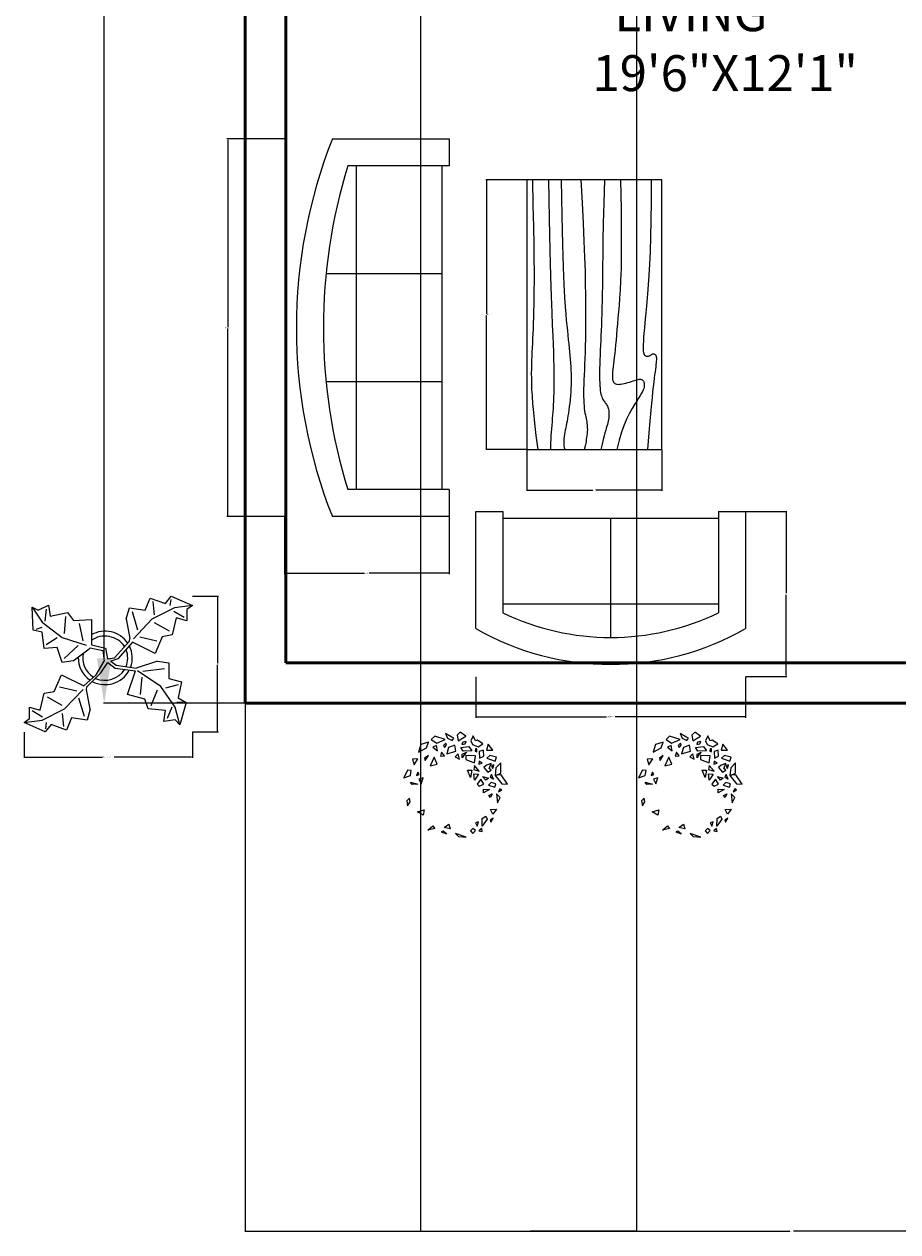
# Model space of a CAD drawing. Units: inches. Extents: x 177 to 602, y 30 to 608.
# Tile 1 of 4: x 204 to 398, y 31 to 299. Entities that reach past the tile are written whole.
import ezdxf

# ---------------------------------------------------------------- set-up
doc = ezdxf.new("R2010")
doc.units = ezdxf.units.IN
doc.header["$MEASUREMENT"] = 0
for name, color, linetype, lineweight in [('A-ANNO-DIMS', 2, 'Continuous', 18), ('A-AREA-IDEN', 7, 'Continuous', 25), ('A-FURN', 8, 'Continuous', 18), ('A-WALL', 7, 'Continuous', 50), ('L-PLNT', 94, 'Continuous', 13)]:
    doc.layers.add(name, color=color, linetype=linetype, lineweight=lineweight)
doc.styles.get("Standard").update_dxf_attribs({"font": 'arial.ttf'})
doc.dimstyles.get("Standard").update_dxf_attribs({"dimtxt": 0.18, "dimasz": 0.18, "dimexe": 0.18, "dimexo": 0.0625, "dimgap": 0.09, "dimtad": 0, "dimtih": 1, "dimtoh": 1, "dimdec": 1, "dimzin": 0, "dimdsep": 46, "dimlunit": 4, "dimtxsty": 'Standard', "dimcen": 0.09, "dimadec": 0, "dimazin": 0, "dimtfac": 1, "dimtdec": 1, "dimtofl": 0, "dimtmove": 0, "dimatfit": 3, "dimfxl": 1, "dimtolj": 1, "dimtzin": 0, "dimarcsym": 0})

# ---------------------------------------------------------------- blocks, each defined once
blk = doc.blocks.new('*U9')
for points in [[(-4.43, 11.05), (-5.18, 10.36), (-3.96, 9.49), (-2.07, 10.36)], [(-2, 11.66), (-1.6, 10.62), (-0.52, 10.1), (-0.18, 10.62), (-0.79, 10.96)], [(1.24, 12), (0.56, 11.31), (0.76, 10.01), (2.52, 11.05)], [(4.14, 11.14), (3.6, 10.01), (4, 9.23), (5.22, 8.71), (6.3, 9.41), (5.08, 10.19), (4.61, 10.01)], [(-5.78, 9.75), (-7.54, 9.23), (-8.01, 7.5), (-6.26, 8.45)], [(-4.84, 8.63), (-3.83, 7.85), (-4.03, 8.97)], [(-1.94, 9.49), (-2.48, 8.97), (-2.27, 8.54), (-1.8, 9.06)], [(0.02, 9.06), (-1.33, 8.54), (-1.73, 7.16), (0.29, 7.76)], [(1.37, 8.54), (3.13, 8.8), (3.8, 7.85), (1.91, 7.76)], [(2.59, 9.93), (1.84, 9.75), (1.64, 9.23), (2.32, 9.41)], [(4.61, 8.28), (4.54, 7.76), (4.95, 7.59), (4.95, 8.28)], [(7.45, 9.32), (7.11, 7.94), (8.52, 7.94)], [(-8.14, 6.03), (-9.36, 5.95), (-9.02, 4.73)], [(-5.78, 6.81), (-6.66, 6.21), (-6.52, 5.69)], [(-4.57, 6.38), (-5.45, 4.47), (-3.89, 4.82)], [(-2.88, 7.5), (-3.15, 6.64), (-2.27, 6.72)], [(0.76, 7.16), (0.09, 6.46), (1.1, 5.95)], [(1.71, 6.29), (1.71, 7.07), (2.65, 7.5), (2.11, 6.9)], [(2.52, 6.81), (2.52, 5.86), (4.41, 5.17), (4.61, 6.72)], [(5.49, 5.51), (5.42, 4.82), (6.16, 5.08)], [(6.43, 7.94), (5.49, 7.68), (5.56, 6.21), (6.5, 6.64)], [(7.85, 6.81), (7.18, 6.21), (9, 5.51), (9.33, 6.38)], [(-11.32, 1.79), (-9.83, 2.31), (-9.63, 3.44), (-10.44, 3.52)], [(-8.21, 3.09), (-8.48, 2.31), (-7.87, 2.57)], [(3.53, 1.88), (2.86, 3.52), (3.8, 3.52)], [(4.41, 4.56), (4.27, 3.7), (5.49, 3.26)], [(4.27, 2.74), (5.29, 2.66), (4.41, 1.27)], [(8.12, 4.99), (7.11, 4.65), (6.5, 4.13), (7.38, 3.09), (8.12, 3.52), (7.65, 3.87)], [(8.73, 4.73), (8.19, 4.56), (8.39, 3.87), (8.59, 4.04)], [(10.28, 5.17), (9.2, 4.04), (9, 2.31), (10.48, 0.49), (11.76, 0.41), (10.35, 2.48), (9.33, 2.4), (10.28, 2.83)], [(-8.21, 0.41), (-9.43, 0.32), (-9.83, 0.84)], [(-7, 1.79), (-7.94, 1.53), (-7.47, 0.49)], [(5.83, 1.53), (5.02, 0.41), (5.49, -0.02), (6.5, 0.41)], [(7.51, 1.71), (6.91, 1.27), (6.23, 2.14)], [(8.12, 0.75), (7.51, 0.15), (8.93, -0.28), (9.13, 0.49)], [(8.19, 2.57), (7.92, 2.05), (8.66, 1.53)], [(7.78, -0.8), (6.43, -1.5), (6.43, -0.72)], [(8.32, -1.75), (7.98, -2.53), (7.58, -2.1)], [(9.33, -1.75), (9.54, -3.74), (10.14, -2.53)], [(10.08, -0.63), (9.74, -1.32), (10.48, -0.89)], [(-10.03, -2.71), (-10.64, -3.31), (-10.44, -4.44), (-9.9, -3.49)], [(-8.28, -5.73), (-6.79, -5.3), (-7, -6.51)], [(9.33, -5.13), (8.46, -6.25), (7.98, -5.22)], [(5.29, -7.98), (4.61, -8.16), (5.02, -8.94)], [(6.1, -8.94), (6.16, -7.21), (6.91, -6.69), (7.24, -7.38)], [(8.05, -8.07), (8.59, -7.12), (7.92, -7.55)], [(-4.84, -8.85), (-4.43, -9.45), (-5.99, -9.8)], [(-2.54, -10.06), (-3.02, -10.23), (-1.8, -10.67)], [(-2.34, -9.2), (-1.26, -8.5), (-0.99, -9.54)], [(0.22, -10.58), (0.83, -11.27), (2.59, -11.36)], [(4.07, -9.45), (3.53, -9.97), (4.07, -10.58), (4.61, -9.89)], [(6.03, -9.45), (5.42, -9.97), (6.16, -10.15)]]:
    blk.add_lwpolyline(points, close=True)
blk = doc.blocks.new('Sofa - Roundback 7 ft.')
for p, q in [((-12.00002, -32.4421), (-12.00003, -6.5971)), ((11.99997, -32.4421), (11.99998, -6.5971)), ((-36.000027, -34), (-36.000027, -11.4696)), ((-35.999844, -13.3819), (35.9998, -13.3819)), ((35.99998, -34), (35.99998, -11.4696)), ((-36.000027, -32.4421), (35.99998, -32.4421))]:
    blk.add_line(p, q)
for points in [[(-36.000027, -34), (-42.000027, -34), (-42.000027, -8)], [(41.99998, -8), (41.99998, -34), (35.99998, -34)]]:
    blk.add_lwpolyline(points)
for centre, radius, start, end in [((0, -114.25), 114.25, 68.43141, 111.5686), ((-0.00001, -127.1968), 121.1968, 72.72033, 107.2797)]:
    blk.add_arc(centre, radius, start, end)
blk = doc.blocks.new('Sofa - Roundback Loveseat 5 ft.')
for p, q in [((0, -32.44198), (0, -5.99998)), ((-24, -33.99998), (-24, -11.46958)), ((-23.9998, -13.38178), (23.99986, -13.38178)), ((24.00004, -33.99998), (24.00004, -11.46958)), ((-24, -32.44198), (24.00004, -32.44198))]:
    blk.add_line(p, q)
for points in [[(-24, -33.99998), (-30, -33.99998), (-30, -7.99998)], [(30.00004, -7.99998), (30.00004, -33.99998), (24.00004, -33.99998)]]:
    blk.add_lwpolyline(points)
for centre, radius, start, end in [((0, -60.24998), 60.24998, 60.13715, 119.8628), ((0, -61.38438), 55.38444, 64.32083, 115.6792)]:
    blk.add_arc(centre, radius, start, end)
blk = doc.blocks.new('Plant - Rubber or Philodendron')
for p, q in [((8.8871, 10.7908), (9.9809, 13.4933)), ((9.9809, 13.4933), (13.3837, 12.301)), ((13.3837, 12.301), (14.68, 13.9039)), ((14.68, 13.9039), (19.3848, 11.8146)), ((-16.2005, 11.4774), (-13.9899, 8.1064)), ((-16.2005, 11.4774), (-14.8639, 10.7964)), ((-16.0159, 6.3329), (-16.2005, 11.4774)), ((-14.8639, 10.7964), (-12.6195, 11.8975)), ((-13.3174, 8.325), (-13.0735, 11.0065)), ((-12.6195, 11.8975), (-12.1909, 9.4345)), ((4.6914, 8.8812), (5.3859, 11.2828)), ((5.3859, 11.2828), (8.8871, 10.7908)), ((15.3859, 11.3055), (10.3916, 8.7942)), ((10.5828, 12.6946), (10.8893, 9.7953)), ((14.5816, 13.2037), (14.3848, 11.8033)), ((19.3848, 11.8146), (15.3859, 11.3055)), ((19.3848, 11.8146), (18.1868, 10.9119)), ((18.1868, 10.9119), (18.1925, 8.4119)), ((-13.9899, 8.1064), (-9.5434, 4.7185)), ((-12.1909, 9.4345), (-8.3829, 10.3)), ((-8.8369, 9.409), (-9.0894, 5.6095)), ((-8.3829, 10.3), (-7.0549, 8.501)), ((-7.0549, 8.501), (-3.0284, 8.6941)), ((-3.0284, 8.6941), (-3.0709, 3.1041)), ((4.6914, 8.8812), (5.5014, 4.4831)), ((5.9878, 10.4842), (7.1971, 6.3869)), ((10.3916, 8.7942), (6.2847, 4.4028)), ((15.7909, 9.1065), (14.8995, 5.3044)), ((15.2875, 10.6053), (17.5907, 9.2105)), ((18.1925, 8.4119), (15.7909, 9.1065)), ((-14.0069, 5.8704), (-16.0159, 6.3329)), ((-15.3434, 6.5514), (-13.9984, 6.9884)), ((-13.5868, 2.2894), (-14.0069, 5.8704)), ((-4.8529, 4.012), (-5.7184, 7.82)), ((14.2977, 6.1031), (10.9934, 7.9956)), ((-13.1329, 3.1804), (-10.6614, 4.727)), ((-9.5434, 4.7185), (-4.1917, 2.9888)), ((-9.1318, 0.0195), (-5.9793, 2.9025)), ((-3.0709, 3.1041), (0.0797, 2.3163)), ((2.1141, 0.2298), (5.4346, 3.9146)), ((6.1032, 3.6844), (2.8262, -0.031)), ((5.4346, 3.9146), (5.5014, 4.4831)), ((11.1089, 1.1958), (6.1032, 3.6844)), ((7.7005, 4.8881), (11.5025, 3.9967)), ((12.7005, 4.8994), (11.1089, 1.1958)), ((14.8995, 5.3044), (12.7005, 4.8994)), ((-10.6784, 2.491), (-13.5868, 2.2894)), ((-9.5858, -0.8715), (-10.6784, 2.491)), ((-7.1228, -0.443), (-3.5248, 2.2131)), ((-3.5248, 2.2131), (-3.3011, 2.4355)), ((-3.3011, 2.4355), (-0.5306, 1.7947)), ((-0.5306, 1.7947), (-0.2255, -0.5527)), ((-0.5306, 1.7947), (-0.5306, 1.7947)), ((0.0797, 2.3163), (0.4866, -0.031)), ((0.4866, -0.031), (2.1141, 0.2298)), ((-7.1228, -0.443), (-9.5858, -0.8715)), ((-2.019, -3.6148), (-0.2255, -0.5527)), ((-0.9375, -3.1608), (0.5883, -0.8135)), ((0.5883, -0.8135), (2.2447, -2.0916)), ((2.8262, -0.031), (1.3003, -0.5527)), ((1.3003, -0.5527), (2.4193, -1.4655)), ((2.2447, -2.0916), (6.7108, -2.6626)), ((2.4193, -1.4655), (6.895, -2.1175)), ((4.943, -7.9659), (6.7108, -2.6626)), ((11.6605, -0.5413), (6.895, -2.1175)), ((12.3677, -6.1981), (7.219, -2.6772)), ((8.3544, -2.7453), (13.1973, -2.1704)), ((11.6605, -0.5413), (14.1354, -0.8948)), ((14.1354, -0.8948), (14.1354, -4.4304)), ((-11.3237, -7.2629), (-9.7321, -3.5593)), ((-9.7321, -3.5593), (-4.7264, -6.0479)), ((-2.019, -3.6148), (-4.7264, -6.0479)), ((-4.0579, -6.2781), (-0.9375, -3.1608)), ((8.125, -4.0768), (7.7715, -7.9659)), ((14.1354, -4.4304), (16.9638, -5.1375)), ((16.9638, -5.1375), (16.2567, -8.673)), ((-14.4141, -11.4699), (-13.5228, -7.6679)), ((-13.5228, -7.6679), (-11.3237, -7.2629)), ((-6.3237, -7.2516), (-10.1257, -6.3602)), ((-9.0148, -11.1577), (-4.9047, -6.8122)), ((-4.1246, -6.8466), (-4.0579, -6.2781)), ((-3.3146, -11.2447), (-4.1246, -6.8466)), ((8.8321, -9.0266), (4.943, -7.9659)), ((10.2463, -10.4408), (11.6605, -6.9053)), ((15.5496, -10.7943), (12.3677, -6.1981)), ((16.2567, -5.8446), (13.4283, -6.5517)), ((-12.921, -8.4665), (-9.6166, -10.359)), ((-4.611, -12.8477), (-5.8203, -8.7504)), ((9.5392, -11.1479), (8.8321, -9.0266)), ((17.3174, -9.7337), (15.9032, -9.7337)), ((16.2567, -8.673), (18.0245, -9.7337)), ((18.0245, -9.7337), (16.6103, -14.6834)), ((-18.008, -14.1781), (-16.8101, -13.2754)), ((-16.8157, -10.7754), (-14.4141, -11.4699)), ((-16.8101, -13.2754), (-16.8157, -10.7754)), ((-13.9107, -12.9688), (-16.2139, -11.574)), ((-14.0091, -13.669), (-9.0148, -11.1577)), ((-9.206, -15.0581), (-9.5126, -12.1588)), ((-7.5103, -13.1543), (-8.6042, -15.8568)), ((-4.0092, -13.6463), (-7.5103, -13.1543)), ((-3.3146, -11.2447), (-4.0092, -13.6463)), ((13.4283, -11.5015), (9.5392, -11.1479)), ((13.0748, -13.9763), (13.4283, -11.5015)), ((14.8425, -10.7943), (13.7819, -13.2692)), ((16.6103, -14.6834), (15.5496, -10.7943)), ((-18.008, -14.1781), (-14.0091, -13.669)), ((-13.3032, -16.2674), (-18.008, -14.1781)), ((-12.0069, -14.6645), (-13.3032, -16.2674)), ((-13.2048, -15.5672), (-13.008, -14.1668)), ((-8.6042, -15.8568), (-12.0069, -14.6645)), ((15.5496, -13.6228), (13.0748, -13.9763)), ((16.6103, -14.6834), (15.5496, -13.6228))]:
    blk.add_line(p, q)
for centre, radius, start, end in [((0, 0), 6.1275, 34.37569, 120.1028), ((-0.0601, -0.2075), 5.2461, 33.82192, 124.9414), ((-0.098, 0.1364), 6.1288, 341.2017, 26.09184), ((0.0308, 0.1664), 6, 178.6147, 235.1169), ((0.0308, 0.1664), 5, 168.1647, 238.6725), ((-0.2664, 0.1682), 5.2775, 338.4094, 20.03007), ((-0.0234, 0.3825), 6.1492, 242.5812, 331.2714), ((-0.1102, 0.4886), 5.2883, 247.3711, 327.472)]:
    blk.add_arc(centre, radius, start, end)
blk = doc.blocks.new('Table - Rectangular Woodgrain 60 x 30 in.')
for p, q in [((0, 0), (0, -30)), ((60, 0), (0, 0)), ((60, -30), (60, 0)), ((0, -30), (60, -30))]:
    blk.add_line(p, q)
for points in [[(0, -2.4), (4.8155, -2.418), (9.0302, -2.4688), (12.709, -2.5477), (15.9167, -2.65), (18.7181, -2.7711), (21.1781, -2.9063), (23.3616, -3.0508), (25.3333, -3.2), (27.1477, -3.3495), (28.8172, -3.4958), (30.3437, -3.636), (31.7291, -3.7667), (32.9756, -3.8849), (34.0849, -3.9875), (35.059, -4.0714), (35.9, -4.1334), (36.6114, -4.1711), (37.2041, -4.1854), (37.6906, -4.1779), (38.0833, -4.15), (38.3948, -4.1034), (38.6375, -4.0396), (38.8239, -3.9602), (38.9666, -3.8667), (39.0764, -3.7608), (39.1573, -3.6448), (39.2116, -3.521), (39.2416, -3.3917), (39.2498, -3.2593), (39.2385, -3.1261), (39.21, -2.9944), (39.1666, -2.8667), (39.111, -2.7447), (39.0468, -2.6281), (38.978, -2.5163), (38.9083, -2.4083), (38.8418, -2.3035), (38.7823, -2.201), (38.7337, -2.1001), (38.7, -2), (38.6844, -1.9003), (38.6875, -1.8021), (38.7094, -1.707), (38.75, -1.6167), (38.8094, -1.5326), (38.8875, -1.4563), (38.9844, -1.3893), (39.1, -1.3333), (39.2351, -1.2896), (39.3937, -1.2583), (39.5804, -1.2396), (39.8, -1.2333), (40.057, -1.2396), (40.3562, -1.2583), (40.7023, -1.2896), (41.1, -1.3333), (41.5547, -1.3895), (42.0755, -1.4573), (42.6721, -1.5361), (43.3542, -1.625), (44.1316, -1.7233), (45.014, -1.8302), (46.0114, -1.9449), (47.1333, -2.0667), (48.3862, -2.1947), (49.7625, -2.3281), (51.2513, -2.4663), (52.8416, -2.6083), (54.5226, -2.7535), (56.2833, -2.9011), (58.1127, -3.0501), (60, -3.2)], [(0, -9.2), (6.5759, -9.0858), (11.9385, -9.0365), (16.2527, -9.0418), (19.6833, -9.0917), (22.3952, -9.1759), (24.5531, -9.2844), (26.322, -9.4069), (27.8666, -9.5333), (29.3241, -9.6553), (30.7203, -9.7719), (32.0532, -9.8837), (33.3208, -9.9917), (34.5213, -10.0965), (35.6526, -10.199), (36.7128, -10.2999), (37.7, -10.4), (38.6129, -10.4996), (39.4531, -10.5969), (40.223, -10.6895), (40.925, -10.775), (41.5613, -10.8512), (42.1344, -10.9156), (42.6465, -10.966), (43.1, -11), (43.4976, -11.0158), (43.8437, -11.0136), (44.143, -10.9942), (44.4, -10.9583), (44.6195, -10.9069), (44.8062, -10.8406), (44.9648, -10.7603), (45.1, -10.6667), (45.2155, -10.5598), (45.3114, -10.4365), (45.3871, -10.2929), (45.4416, -10.125), (45.4743, -9.929), (45.4844, -9.7011), (45.4709, -9.4371), (45.4333, -9.1333), (45.3716, -8.7883), (45.2896, -8.4104), (45.1919, -8.0107), (45.0833, -7.6), (44.9685, -7.1893), (44.8521, -6.7896), (44.7388, -6.4117), (44.6333, -6.0667), (44.54, -5.7628), (44.4614, -5.4979), (44.4001, -5.2675), (44.3583, -5.0667), (44.3384, -4.8909), (44.3427, -4.7354), (44.3736, -4.5956), (44.4333, -4.4667), (44.5236, -4.3453), (44.6427, -4.2333), (44.7884, -4.1339), (44.9583, -4.05), (45.1501, -3.9849), (45.3614, -3.9417), (45.59, -3.9234), (45.8333, -3.9333), (46.0915, -3.9749), (46.3734, -4.0531), (46.6906, -4.1736), (47.0542, -4.3417), (47.4756, -4.5629), (47.9661, -4.8427), (48.5372, -5.1866), (49.2, -5.6), (49.9676, -6.0844), (50.8594, -6.625), (51.8965, -7.2031), (53.1, -7.8), (54.491, -8.3969), (56.0906, -8.975), (57.9199, -9.5156), (60, -10)], [(0, -12.8), (5.1847, -12.9322), (9.6213, -13.0323), (13.3963, -13.1059), (16.5958, -13.1583), (19.3063, -13.1952), (21.614, -13.2219), (23.6054, -13.2439), (25.3666, -13.2667), (26.9728, -13.2947), (28.4531, -13.3281), (29.8256, -13.3663), (31.1083, -13.4083), (32.3191, -13.4535), (33.476, -13.501), (34.597, -13.5501), (35.7, -13.6), (36.7984, -13.6497), (37.8875, -13.6979), (38.9578, -13.743), (40, -13.7833), (41.0047, -13.8174), (41.9625, -13.8438), (42.864, -13.8607), (43.7, -13.8667), (44.4631, -13.8604), (45.1552, -13.8417), (45.7801, -13.8104), (46.3416, -13.7667), (46.8439, -13.7104), (47.2906, -13.6417), (47.6858, -13.5604), (48.0333, -13.4667), (48.3375, -13.3608), (48.6042, -13.2448), (48.8396, -13.121), (49.05, -12.9917), (49.2417, -12.8593), (49.4208, -12.7261), (49.5937, -12.5944), (49.7667, -12.4667), (49.9452, -12.3451), (50.1323, -12.2313), (50.3303, -12.1268), (50.5416, -12.0333), (50.7686, -11.9524), (51.0135, -11.8854), (51.2788, -11.8341), (51.5666, -11.8), (51.8785, -11.7843), (52.2116, -11.7865), (52.562, -11.8059), (52.926, -11.8417), (53.2998, -11.8931), (53.6795, -11.9594), (54.0614, -12.0397), (54.4416, -12.1333), (54.8223, -12.2401), (55.2293, -12.3625), (55.6942, -12.5037), (56.2489, -12.6667), (56.9251, -12.8547), (57.7545, -13.0708), (58.7689, -13.3182), (60, -13.6)], [(0, -18), (5.124, -17.7273), (9.6609, -17.5057), (13.6705, -17.3303), (17.2125, -17.1958), (20.3467, -17.0973), (23.1328, -17.0297), (25.6307, -16.9878), (27.9, -16.9667), (29.9928, -16.9617), (31.9302, -16.9703), (33.7254, -16.9907), (35.3917, -17.0208), (36.9423, -17.0588), (38.3906, -17.1026), (39.7499, -17.1503), (41.0333, -17.2), (42.2519, -17.2496), (43.4073, -17.2969), (44.4986, -17.3395), (45.525, -17.375), (46.4858, -17.4012), (47.3802, -17.4156), (48.2074, -17.416), (48.9667, -17.4), (49.6583, -17.3662), (50.2872, -17.3167), (50.8595, -17.2547), (51.3812, -17.1833), (51.8584, -17.1057), (52.2971, -17.025), (52.7034, -16.9443), (53.0833, -16.8667), (53.443, -16.7951), (53.789, -16.7313), (54.128, -16.6768), (54.4666, -16.6334), (54.8115, -16.6024), (55.1693, -16.5854), (55.5465, -16.5841), (55.95, -16.6), (56.3828, -16.6337), (56.8346, -16.6823), (57.2915, -16.7418), (57.7396, -16.8084), (58.165, -16.878), (58.5539, -16.9469), (58.8924, -17.0111), (59.1666, -17.0667), (59.3679, -17.1107), (59.5078, -17.1438), (59.6032, -17.1675), (59.6708, -17.1833), (59.7275, -17.193), (59.7901, -17.1979), (59.8753, -17.1998), (60, -17.2)], [(0, -22.4), (8.0098, -22.2501), (14.4094, -22.1011), (19.4168, -21.9535), (23.25, -21.8083), (26.1269, -21.6663), (28.2656, -21.5281), (29.884, -21.3947), (31.2, -21.2667), (32.3967, -21.1448), (33.5172, -21.0292), (34.5697, -20.9198), (35.5625, -20.8167), (36.5037, -20.7198), (37.4015, -20.6292), (38.2642, -20.5448), (39.1, -20.4667), (39.9164, -20.3951), (40.7187, -20.3313), (41.5117, -20.2768), (42.3, -20.2333), (43.0883, -20.2024), (43.8812, -20.1854), (44.6836, -20.1841), (45.5, -20.2), (46.3328, -20.234), (47.1747, -20.2844), (48.0163, -20.3488), (48.8479, -20.425), (49.66, -20.5106), (50.4429, -20.6031), (51.1872, -20.7004), (51.8833, -20.8), (52.5246, -20.8999), (53.1166, -20.9995), (53.6681, -21.0983), (54.1875, -21.1958), (54.6834, -21.2919), (55.1646, -21.3859), (55.6394, -21.4777), (56.1167, -21.5667), (56.6028, -21.6515), (57.0961, -21.7266), (57.5929, -21.7852), (58.0896, -21.8208), (58.5823, -21.8268), (59.0674, -21.7964), (59.5412, -21.723), (60, -21.6)], [(0, -25.2), (8.6355, -25.0504), (15.7026, -24.9031), (21.4049, -24.7606), (25.9458, -24.625), (29.529, -24.4988), (32.3578, -24.3844), (34.6359, -24.284), (36.5667, -24.2), (38.3213, -24.1341), (39.9417, -24.0854), (41.437, -24.0523), (42.8167, -24.0333), (44.0901, -24.0268), (45.2667, -24.0313), (46.3557, -24.0451), (47.3667, -24.0667), (48.309, -24.0947), (49.1928, -24.1287), (50.0284, -24.168), (50.826, -24.2125), (51.5959, -24.2617), (52.3483, -24.3151), (53.0935, -24.3725), (53.8417, -24.4334), (54.6009, -24.497), (55.3699, -24.561), (56.1454, -24.6226), (56.9239, -24.6792), (57.7021, -24.7279), (58.4764, -24.7662), (59.2435, -24.7911), (60, -24.8)], [(0, -28.8), (5.6867, -28.6681), (10.45, -28.5698), (14.407, -28.5012), (17.675, -28.4584), (20.3711, -28.4374), (22.6125, -28.4344), (24.5164, -28.4455), (26.2, -28.4667), (27.762, -28.4947), (29.2276, -28.5281), (30.6033, -28.5663), (31.8958, -28.6084), (33.1118, -28.6535), (34.2578, -28.7011), (35.3405, -28.7501), (36.3666, -28.8), (37.3443, -28.8497), (38.288, -28.8974), (39.2137, -28.9412), (40.1375, -28.9792), (41.0753, -29.0093), (42.0432, -29.0297), (43.0572, -29.0384), (44.1333, -29.0333), (45.2936, -29.0114), (46.5843, -28.9641), (48.0579, -28.8816), (49.7666, -28.7542), (51.7629, -28.5721), (54.0989, -28.3255), (56.8272, -28.0048), (60, -27.6)]]:
    blk.add_lwpolyline(points)
blk = doc.blocks.new('*D33')
at = {"layer": 'A-ANNO-DIMS', "color": 0, "lineweight": -2, "transparency": 16777216}
for p, q in [((253.28, 556.14), (221.81, 556.14)), ((221.99, 546.14), (221.99, 358.36)), ((221.99, 158.14), (221.99, 345.92)), ((253.28, 148.14), (221.81, 148.14))]:
    blk.add_line(p, q, dxfattribs=at)
at = {"layer": 'A-ANNO-DIMS', "color": 0, "transparency": 16777216}
for points in [[(220.33, 546.14), (223.66, 546.14), (221.99, 556.14)], [(220.33, 158.14), (223.66, 158.14), (221.99, 148.14)]]:
    blk.add_solid(points, dxfattribs=at)
at = {"layer": 'Defpoints', "color": 0, "transparency": 16777216}
for p in [(221.99, 556.14), (253.34, 556.14), (253.34, 148.14)]:
    blk.add_point(p, dxfattribs=at)
at = {"layer": 'A-ANNO-DIMS', "color": 0, "transparency": 16777216, "insert": (221.99, 352.14), "char_height": 12, "attachment_point": 5}
blk.add_mtext("\\A1;34'", dxfattribs=at)
blk = doc.blocks.new('*D41')
at = {"layer": 'A-ANNO-DIMS', "color": 0, "lineweight": -2, "transparency": 16777216}
for p, q in [((204.2, 141.69), (204.2, 135.96)), ((241.59, 141.69), (241.59, 135.96)), ((204.38, 136.14), (221.61, 136.14)), ((241.41, 136.14), (224.18, 136.14))]:
    blk.add_line(p, q, dxfattribs=at)
at = {"layer": 'A-ANNO-DIMS', "color": 0, "transparency": 16777216}
for points in [[(204.38, 136.17), (204.38, 136.11), (204.2, 136.14)], [(241.41, 136.17), (241.41, 136.11), (241.59, 136.14)]]:
    blk.add_solid(points, dxfattribs=at)
at = {"layer": 'Defpoints', "color": 0, "transparency": 16777216}
for p in [(204.2, 141.75), (241.59, 141.75), (241.59, 136.14)]:
    blk.add_point(p, dxfattribs=at)
at = {"layer": 'A-ANNO-DIMS', "color": 0, "transparency": 16777216, "insert": (222.89, 136.14), "char_height": 0.18, "attachment_point": 5}
blk.add_mtext('\\A1;PLANT 3\'-1 1/2" TYP.', dxfattribs=at)
blk = doc.blocks.new('*D42')
at = {"layer": 'A-ANNO-DIMS', "color": 0, "lineweight": -2, "transparency": 16777216}
for p, q in [((241.65, 171.92), (247.38, 171.92)), ((247.2, 171.74), (247.2, 157.02)), ((247.2, 141.93), (247.2, 156.65)), ((241.65, 141.75), (247.38, 141.75))]:
    blk.add_line(p, q, dxfattribs=at)
at = {"layer": 'A-ANNO-DIMS', "color": 0, "transparency": 16777216}
for points in [[(247.17, 171.74), (247.23, 171.74), (247.2, 171.92)], [(247.17, 141.93), (247.23, 141.93), (247.2, 141.75)]]:
    blk.add_solid(points, dxfattribs=at)
at = {"layer": 'Defpoints', "color": 0, "transparency": 16777216}
for p in [(241.59, 171.92), (247.2, 171.92), (241.59, 141.75)]:
    blk.add_point(p, dxfattribs=at)
at = {"layer": 'A-ANNO-DIMS', "color": 0, "transparency": 16777216, "insert": (247.2, 156.84), "char_height": 0.18, "attachment_point": 5}
blk.add_mtext('\\A1;2\'-6" TYP.', dxfattribs=at)
blk = doc.blocks.new('*D57')
at = {"layer": 'A-ANNO-DIMS', "color": 0, "lineweight": -2, "transparency": 16777216}
for p, q in [((261.98, 273.62), (249.26, 273.62)), ((249.44, 273.44), (249.44, 231.8)), ((249.44, 189.8), (249.44, 231.43)), ((261.98, 189.62), (249.26, 189.62))]:
    blk.add_line(p, q, dxfattribs=at)
at = {"layer": 'A-ANNO-DIMS', "color": 0, "transparency": 16777216}
for points in [[(249.41, 273.44), (249.47, 273.44), (249.44, 273.62)], [(249.41, 189.8), (249.47, 189.8), (249.44, 189.62)]]:
    blk.add_solid(points, dxfattribs=at)
at = {"layer": 'Defpoints', "color": 0, "transparency": 16777216}
for p in [(249.44, 273.62), (262.04, 273.62), (262.04, 189.62)]:
    blk.add_point(p, dxfattribs=at)
at = {"layer": 'A-ANNO-DIMS', "color": 0, "transparency": 16777216, "insert": (249.44, 231.62), "char_height": 0.18, "attachment_point": 5}
blk.add_mtext('\\A1;SOFA 7\'-0"', dxfattribs=at)
blk = doc.blocks.new('*D58')
at = {"layer": 'A-ANNO-DIMS', "color": 0, "lineweight": -2, "transparency": 16777216}
for p, q in [((262.04, 189.55), (262.04, 176.84)), ((298.71, 189.55), (298.71, 176.84)), ((262.22, 177.02), (279.84, 177.02)), ((298.53, 177.02), (280.92, 177.02))]:
    blk.add_line(p, q, dxfattribs=at)
at = {"layer": 'A-ANNO-DIMS', "color": 0, "transparency": 16777216}
for points in [[(262.22, 177.05), (262.22, 176.99), (262.04, 177.02)], [(298.53, 177.05), (298.53, 176.99), (298.71, 177.02)]]:
    blk.add_solid(points, dxfattribs=at)
at = {"layer": 'Defpoints', "color": 0, "transparency": 16777216}
for p in [(262.04, 189.62), (298.71, 189.62), (262.04, 177.02)]:
    blk.add_point(p, dxfattribs=at)
at = {"layer": 'A-ANNO-DIMS', "color": 0, "transparency": 16777216, "insert": (280.38, 177.02), "char_height": 0.18, "attachment_point": 5}
blk.add_mtext('\\A1;3\'-0 1/2"', dxfattribs=at)
blk = doc.blocks.new('*D59')
at = {"layer": 'A-ANNO-DIMS', "color": 0, "lineweight": -2, "transparency": 16777216}
for p, q in [((304.58, 154.02), (304.58, 144.9)), ((364.58, 154.02), (364.58, 144.9)), ((304.76, 145.08), (333.56, 145.08)), ((364.4, 145.08), (335.61, 145.08))]:
    blk.add_line(p, q, dxfattribs=at)
at = {"layer": 'A-ANNO-DIMS', "color": 0, "transparency": 16777216}
for points in [[(304.76, 145.11), (304.76, 145.05), (304.58, 145.08)], [(364.4, 145.11), (364.4, 145.05), (364.58, 145.08)]]:
    blk.add_solid(points, dxfattribs=at)
at = {"layer": 'Defpoints', "color": 0, "transparency": 16777216}
for p in [(304.58, 154.08), (364.58, 154.08), (304.58, 145.08)]:
    blk.add_point(p, dxfattribs=at)
at = {"layer": 'A-ANNO-DIMS', "color": 0, "transparency": 16777216, "insert": (334.58, 145.08), "char_height": 0.18, "attachment_point": 5}
blk.add_mtext('\\A1;LOVESEAT 5\'-0"', dxfattribs=at)
blk = doc.blocks.new('*D60')
at = {"layer": 'A-ANNO-DIMS', "color": 0, "lineweight": -2, "transparency": 16777216}
for p, q in [((364.65, 190.75), (373.76, 190.75)), ((373.58, 190.57), (373.58, 172.6)), ((373.58, 154.26), (373.58, 172.23)), ((364.65, 154.08), (373.76, 154.08))]:
    blk.add_line(p, q, dxfattribs=at)
at = {"layer": 'A-ANNO-DIMS', "color": 0, "transparency": 16777216}
for points in [[(373.55, 190.57), (373.61, 190.57), (373.58, 190.75)], [(373.55, 154.26), (373.61, 154.26), (373.58, 154.08)]]:
    blk.add_solid(points, dxfattribs=at)
at = {"layer": 'Defpoints', "color": 0, "transparency": 16777216}
for p in [(364.58, 190.75), (364.58, 154.08), (373.58, 154.08)]:
    blk.add_point(p, dxfattribs=at)
at = {"layer": 'A-ANNO-DIMS', "color": 0, "transparency": 16777216, "insert": (373.58, 172.41), "char_height": 0.18, "attachment_point": 5}
blk.add_mtext('\\A1;3\'-0 1/2"', dxfattribs=at)
blk = doc.blocks.new('*D69')
at = {"layer": 'A-ANNO-DIMS', "color": 0, "lineweight": -2, "transparency": 16777216}
for p, q in [((315.92, 264.53), (306.8, 264.53)), ((306.98, 264.35), (306.98, 234.71)), ((306.98, 204.71), (306.98, 234.35)), ((315.92, 204.53), (306.8, 204.53))]:
    blk.add_line(p, q, dxfattribs=at)
at = {"layer": 'A-ANNO-DIMS', "color": 0, "transparency": 16777216}
for points in [[(306.95, 264.35), (307.01, 264.35), (306.98, 264.53)], [(306.95, 204.71), (307.01, 204.71), (306.98, 204.53)]]:
    blk.add_solid(points, dxfattribs=at)
at = {"layer": 'Defpoints', "color": 0, "transparency": 16777216}
for p in [(315.98, 264.53), (306.98, 204.53), (315.98, 204.53)]:
    blk.add_point(p, dxfattribs=at)
at = {"layer": 'A-ANNO-DIMS', "color": 0, "transparency": 16777216, "insert": (306.98, 234.53), "char_height": 0.18, "attachment_point": 5}
blk.add_mtext('\\A1;COFFEE TABLE 5\'-0"', dxfattribs=at)
blk = doc.blocks.new('*D70')
at = {"layer": 'A-ANNO-DIMS', "color": 0, "lineweight": -2, "transparency": 16777216}
for p, q in [((315.98, 204.47), (315.98, 195.35)), ((345.98, 204.47), (345.98, 195.35)), ((316.16, 195.53), (330.65, 195.53)), ((345.8, 195.53), (331.31, 195.53))]:
    blk.add_line(p, q, dxfattribs=at)
at = {"layer": 'A-ANNO-DIMS', "color": 0, "transparency": 16777216}
for points in [[(316.16, 195.56), (316.16, 195.5), (315.98, 195.53)], [(345.8, 195.56), (345.8, 195.5), (345.98, 195.53)]]:
    blk.add_solid(points, dxfattribs=at)
at = {"layer": 'Defpoints', "color": 0, "transparency": 16777216}
for p in [(315.98, 204.53), (345.98, 204.53), (345.98, 195.53)]:
    blk.add_point(p, dxfattribs=at)
at = {"layer": 'A-ANNO-DIMS', "color": 0, "transparency": 16777216, "insert": (330.98, 195.53), "char_height": 0.18, "attachment_point": 5}
blk.add_mtext('\\A1;2\'-6"', dxfattribs=at)
blk = doc.blocks.new('*D73')
at = {"layer": 'A-ANNO-DIMS', "color": 0, "lineweight": -2, "transparency": 16777216}
for p, q in [((253.34, 148.07), (253.34, 30.54)), ((496.34, 128.07), (496.34, 30.54)), ((253.52, 30.72), (374.44, 30.72)), ((496.16, 30.72), (375.24, 30.72))]:
    blk.add_line(p, q, dxfattribs=at)
at = {"layer": 'A-ANNO-DIMS', "color": 0, "transparency": 16777216}
for points in [[(253.52, 30.75), (253.52, 30.69), (253.34, 30.72)], [(496.16, 30.75), (496.16, 30.69), (496.34, 30.72)]]:
    blk.add_solid(points, dxfattribs=at)
at = {"layer": 'Defpoints', "color": 0, "transparency": 16777216}
for p in [(253.34, 148.14), (496.34, 128.14), (496.34, 30.72)]:
    blk.add_point(p, dxfattribs=at)
at = {"layer": 'A-ANNO-DIMS', "color": 0, "transparency": 16777216, "insert": (374.84, 30.72), "char_height": 0.18, "attachment_point": 5}
blk.add_mtext('\\A1;20\'-3"', dxfattribs=at)
blk = doc.blocks.new('*D85')
at = {"layer": 'A-ANNO-DIMS', "color": 0, "lineweight": -2, "transparency": 16777216}
for p, q in [((292.34, 445.07), (292.34, 30.54)), ((340.34, 445.07), (340.34, 30.54)), ((292.52, 30.72), (316.01, 30.72)), ((340.16, 30.72), (316.67, 30.72))]:
    blk.add_line(p, q, dxfattribs=at)
at = {"layer": 'A-ANNO-DIMS', "color": 0, "transparency": 16777216}
for points in [[(292.52, 30.75), (292.52, 30.69), (292.34, 30.72)], [(340.16, 30.75), (340.16, 30.69), (340.34, 30.72)]]:
    blk.add_solid(points, dxfattribs=at)
at = {"layer": 'Defpoints', "color": 0, "transparency": 16777216}
for p in [(292.34, 445.14), (340.34, 445.14), (340.34, 30.72)]:
    blk.add_point(p, dxfattribs=at)
at = {"layer": 'A-ANNO-DIMS', "color": 0, "transparency": 16777216, "insert": (316.34, 30.72), "char_height": 0.18, "attachment_point": 5}
blk.add_mtext('\\A1;4\'-0"', dxfattribs=at)

msp = doc.modelspace()

# ---------------------------------------------------------------- linework, layer by layer
at = {"layer": 'A-WALL'}
for p, q in [((253.34, 148.14), (253.34, 556.14)), ((262.34, 157.14), (262.34, 439.14)), ((458.08, 157.14), (262.34, 157.14)), ((457.81, 148.14), (253.34, 148.14))]:
    msp.add_line(p, q, dxfattribs=at)

# ---------------------------------------------------------------- block references
at = {"layer": 'A-FURN'}
for name, p, rotation in [('Sofa - Roundback 7 ft.', (264.71, 231.62), 90), ('Table - Rectangular Woodgrain 60 x 30 in.', (345.98, 264.53), 270), ('Sofa - Roundback Loveseat 5 ft.', (334.58, 156.75), 180)]:
    msp.add_blockref(name, p, dxfattribs=dict(at, rotation=rotation))
at = {"layer": 'L-PLNT'}
for name, p in [('Plant - Rubber or Philodendron', (222.2, 158.02)), ('*U9', (299.89, 129.71)), ('*U9', (352.07, 129.71))]:
    msp.add_blockref(name, p, dxfattribs=at)

# ---------------------------------------------------------------- texts
at = {"layer": 'A-AREA-IDEN', "insert": (330.54, 305.6), "char_height": 8, "attachment_point": 1}
msp.add_mtext_dynamic_manual_height_columns('  LIVING\\P19\'6"X12\'1"', width=62.7486, gutter_width=1, heights=[0], dxfattribs=at)

# ---------------------------------------------------------------- dimensions: what is measured, and where the dimension line sits
at = {"layer": 'A-ANNO-DIMS'}
for base, p1, p2, angle, override, picture, middle in [((221.99, 556.14), (253.34, 148.14), (253.34, 556.14), 90, {"dimtxt": 12, "dimasz": 10, "dimclrd": 0, "dimclre": 0, "dimclrt": 0}, '*D33', (221.99, 352.14)), ((373.58, 154.08), (364.58, 190.75), (364.58, 154.08), 270, {"dimdec": 1, "dimlfac": 1, "dimrnd": 0, "dimzin": 1, "dimdsep": 46, "dimlunit": 4, "dimfrac": 2}, '*D60', (373.58, 172.41)), ((262.04, 177.02), (298.71, 189.62), (262.04, 189.62), 180, {"dimdec": 1, "dimlfac": 1, "dimrnd": 0, "dimzin": 1, "dimdsep": 46, "dimlunit": 4, "dimfrac": 2}, '*D58', (280.38, 177.02))]:
    dim = msp.add_linear_dim(base=base, p1=p1, p2=p2, angle=angle, dimstyle='Standard', override=override, dxfattribs=at)
    dim.commit()
    dim.dimension.update_dxf_attribs({"geometry": picture, "text_midpoint": middle})
for base, p1, p2, picture, middle in [((340.34, 30.72), (292.34, 445.14), (340.34, 445.14), '*D85', (316.34, 30.72)), ((345.98, 195.53), (315.98, 204.53), (345.98, 204.53), '*D70', (330.98, 195.53)), ((496.34, 30.72), (253.34, 148.14), (496.34, 128.14), '*D73', (374.84, 30.72))]:
    dim = msp.add_linear_dim(base=base, p1=p1, p2=p2, dimstyle='Standard', override={"dimdec": 1, "dimlfac": 1, "dimrnd": 0, "dimzin": 1, "dimdsep": 46, "dimlunit": 4, "dimfrac": 2}, dxfattribs=at)
    dim.commit()
    dim.dimension.update_dxf_attribs({"geometry": picture, "text_midpoint": middle})
for base, p1, p2, angle, text, picture, middle in [((249.44, 273.62), (262.04, 189.62), (262.04, 273.62), 90, 'SOFA <>', '*D57', (249.44, 231.62)), ((306.98, 204.53), (315.98, 264.53), (315.98, 204.53), 270, 'COFFEE TABLE <>', '*D69', (306.98, 234.53)), ((247.2, 171.92), (241.59, 141.75), (241.59, 171.92), 90, '<> TYP.', '*D42', (247.2, 156.84)), ((304.58, 145.08), (364.58, 154.08), (304.58, 154.08), 180, 'LOVESEAT <>', '*D59', (334.58, 145.08))]:
    dim = msp.add_linear_dim(base=base, p1=p1, p2=p2, angle=angle, text=text, dimstyle='Standard', override={"dimdec": 1, "dimlfac": 1, "dimrnd": 0, "dimzin": 1, "dimdsep": 46, "dimlunit": 4, "dimfrac": 2}, dxfattribs=at)
    dim.commit()
    dim.dimension.update_dxf_attribs({"geometry": picture, "text_midpoint": middle})
dim = msp.add_linear_dim(base=(241.59, 136.14), p1=(204.2, 141.75), p2=(241.59, 141.75), text='PLANT <> TYP.', dimstyle='Standard', override={"dimdec": 1, "dimlfac": 1, "dimrnd": 0, "dimzin": 1, "dimdsep": 46, "dimlunit": 4, "dimfrac": 2}, dxfattribs=at)
dim.commit()
dim.dimension.update_dxf_attribs({"geometry": '*D41', "text_midpoint": (222.89, 136.14)})

doc.saveas('drawing.dxf')
